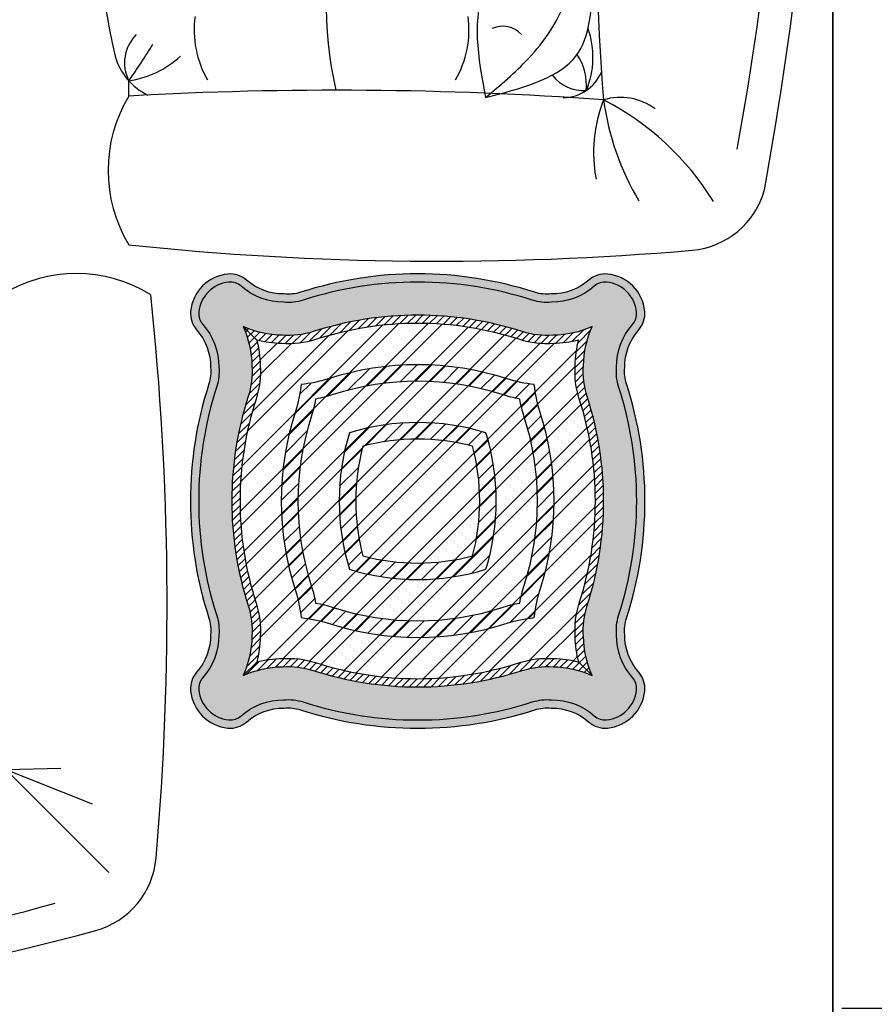
# Model space of a CAD drawing. Units: inches. Extents: x 844 to 2234, y 346 to 1084.
# Tile 67 of 93: x 2014.41 to 2030.9, y 668.63 to 687.63. Entities that reach past the tile are written whole.
import ezdxf

# ---------------------------------------------------------------- set-up
doc = ezdxf.new("R2010")
doc.units = ezdxf.units.IN
doc.header["$MEASUREMENT"] = 0
for name, color, linetype, lineweight in [('A-ANNO-DIMS', 2, 'Continuous', 18), ('A-WALL', 7, 'Continuous', 35), ('furniture', 8, 'Continuous', 18)]:
    doc.layers.add(name, color=color, linetype=linetype, lineweight=lineweight)
for name, color, linetype in [('RA-AP-01$0$FURN', 3, 'Continuous'), ('RA-AP-01$0$steel', 193, 'Continuous'), ('RA-AP-01$0$WOOD', 64, 'Continuous')]:
    doc.layers.add(name, color=color, linetype=linetype)
doc.styles.get("Standard").update_dxf_attribs({"font": 'arial.ttf'})
doc.dimstyles.get("Standard").update_dxf_attribs({"dimtxt": 6, "dimasz": 3, "dimexe": 0.18, "dimexo": 0.0625, "dimgap": 0.09, "dimtad": 0, "dimtih": 1, "dimtoh": 1, "dimdec": 1, "dimzin": 0, "dimdsep": 46, "dimlunit": 3, "dimtxsty": 'Standard', "dimblk": 'ARCHTICK', "dimcen": 0.09, "dimadec": 0, "dimazin": 0, "dimtfac": 1, "dimtdec": 1, "dimtofl": 0, "dimtmove": 0, "dimatfit": 3, "dimfxl": 1, "dimtolj": 1, "dimtzin": 0, "dimarcsym": 0})
pattern_1 = [(45, (0, 1.362436106329781), (-0.0088388347648318, 0.0088388347648318), [])]
pattern_2 = [(45, (0, 1.362436106329781), (-0.0044194173824159, 0.0044194173824159), [])]

# ---------------------------------------------------------------- blocks, each defined once
blk = doc.blocks.new('A$C2FCF5309')
at = {"layer": 'RA-AP-01$0$FURN'}
h = blk.add_hatch(dxfattribs=at)
h.set_pattern_fill('ANSI31', color=256, scale=0.1, style=0)
h.set_pattern_definition(pattern_1)
h.paths.add_polyline_path([(5.038683893313746, -5.169250834004607, -0.1583983521602212), (5.038683893312098, -5.373464580902012, 0.0306258898943267), (5.033304057242972, -5.394827569605182, 0.0306258898948892), (5.01194106853941, -5.40020740567441, -0.1028142994996694), (4.878286182323899, -5.414871334512708), (4.863600873530158, -5.43331743520547, 0.1120482678681049), (5.018059823131753, -5.419248541734471, -0.052642197802937), (5.050972078299936, -5.412495590662115, -0.0526421977994963), (5.057725029371615, -5.379583335496025, 0.1583028414702701), (5.057725029372958, -5.163132079409654, -0.052642197806903), (5.050972078299777, -5.130219824239078, -0.0526421977995126), (5.018059823133679, -5.123466873167369, 0.0215995840215353), (4.988903013548211, -5.115372132362452), (4.975007495303644, -5.132826183367946, -0.0289147572844802), (5.011941068537408, -5.142508009226167, 0.0306258898976746), (5.033304057242868, -5.147887845296027, 0.0306258899022411)])
h.paths.add_polyline_path([(4.975007495303645, -5.132826183367946), (4.988903013548211, -5.115372132362452, 0.1362374241599938), (4.801608567045604, -5.12346687316654, -0.0526421978036853), (4.768696311876971, -5.130219824239102, -0.05264219780204), (4.761943360804856, -5.163132079406747, 0.1583028414743723), (4.761943360806116, -5.379583335498449, -0.0526421977955461), (4.768696311877141, -5.412495590662114, -0.0526421978073986), (4.801608567048022, -5.419248541735437, 0.0454484293938888), (4.863600873530158, -5.43331743520547), (4.878286182323899, -5.414871334512708, -0.0546933379798044), (4.80772732164382, -5.40020740567649, 0.030625889903973), (4.786364332934043, -5.394827569605216, 0.0306258898932853), (4.780984496865101, -5.373464580902791, -0.1583983521638281), (4.780984496864308, -5.169250834000963, 0.03062588989692), (4.786364332933943, -5.147887845296004, 0.0306258898946324), (4.807727321637318, -5.142508009226805, -0.1288932573266927)])
h.paths.add_polyline_path([(4.843422214712861, -5.204945727074827, -0.0783685831716868), (4.924134454130224, -5.196727409635105), (4.939146578618322, -5.177870798323143, 0.1012675676854134), (4.827248748758957, -5.188772261120899, 0.1253648873081696), (4.820394258584192, -5.327034652050361), (4.837127701354095, -5.306015906404253, -0.0981593964869636)], flags=17)
h.paths.add_polyline_path([(4.843422214712824, -5.337769687826355, -0.0311091841722656), (4.837127701354095, -5.306015906404253), (4.820394258584193, -5.32703465205036, 0.0247727657431944), (4.827248748758908, -5.353943153780261, 0.0812754385032542), (4.916962478476905, -5.36629034358622), (4.933684093813825, -5.345286454285511, -0.0876255421014372)], flags=17)
h.paths.add_polyline_path([(4.992419641418037, -5.353943153780226, 0.1506053783834298), (4.992419641417933, -5.188772261120954, 0.0485966419124224), (4.939146578618321, -5.177870798323143), (4.924134454130224, -5.196727409635105, -0.0507799419579301), (4.976246175464031, -5.204945727074882, -0.1296645318906876), (4.97624617546411, -5.337769687826316, -0.0415667119298777), (4.933684093813825, -5.345286454285511), (4.916962478476905, -5.36629034358622, 0.0684915676023693)], flags=17)
h = blk.add_hatch(dxfattribs=at)
h.set_pattern_fill('ANSI31', color=256, scale=0.1, style=0)
h.set_pattern_definition(pattern_1)
h.paths.add_polyline_path([(5.038683893313746, -5.169250834004607, -0.1583983521602212), (5.038683893312098, -5.373464580902012, 0.0306258898943267), (5.033304057242972, -5.394827569605182, 0.0306258898948892), (5.01194106853941, -5.40020740567441, -0.1028142994996694), (4.878286182323899, -5.414871334512708), (4.863600873530158, -5.43331743520547, 0.1120482678681049), (5.018059823131753, -5.419248541734471, -0.052642197802937), (5.050972078299936, -5.412495590662115, -0.0526421977994963), (5.057725029371615, -5.379583335496025, 0.1583028414702701), (5.057725029372958, -5.163132079409654, -0.052642197806903), (5.050972078299777, -5.130219824239078, -0.0526421977995126), (5.018059823133679, -5.123466873167369, 0.0215995840215353), (4.988903013548211, -5.115372132362452), (4.975007495303644, -5.132826183367946, -0.0289147572844802), (5.011941068537408, -5.142508009226167, 0.0306258898976746), (5.033304057242868, -5.147887845296027, 0.0306258899022411)])
h.paths.add_polyline_path([(4.975007495303645, -5.132826183367946), (4.988903013548211, -5.115372132362452, 0.1362374241599938), (4.801608567045604, -5.12346687316654, -0.0526421978036853), (4.768696311876971, -5.130219824239102, -0.05264219780204), (4.761943360804856, -5.163132079406747, 0.1583028414743723), (4.761943360806116, -5.379583335498449, -0.0526421977955461), (4.768696311877141, -5.412495590662114, -0.0526421978073986), (4.801608567048022, -5.419248541735437, 0.0454484293938888), (4.863600873530158, -5.43331743520547), (4.878286182323899, -5.414871334512708, -0.0546933379798044), (4.80772732164382, -5.40020740567649, 0.030625889903973), (4.786364332934043, -5.394827569605216, 0.0306258898932853), (4.780984496865101, -5.373464580902791, -0.1583983521638281), (4.780984496864308, -5.169250834000963, 0.03062588989692), (4.786364332933943, -5.147887845296004, 0.0306258898946324), (4.807727321637318, -5.142508009226805, -0.1288932573266927)])
h.paths.add_polyline_path([(4.843422214712861, -5.204945727074827, -0.0783685831716868), (4.924134454130224, -5.196727409635105), (4.939146578618322, -5.177870798323143, 0.1012675676854134), (4.827248748758957, -5.188772261120899, 0.1253648873081696), (4.820394258584192, -5.327034652050361), (4.837127701354095, -5.306015906404253, -0.0981593964869636)], flags=17)
h.paths.add_polyline_path([(4.843422214712824, -5.337769687826355, -0.0311091841722656), (4.837127701354095, -5.306015906404253), (4.820394258584193, -5.32703465205036, 0.0247727657431944), (4.827248748758908, -5.353943153780261, 0.0812754385032542), (4.916962478476905, -5.36629034358622), (4.933684093813825, -5.345286454285511, -0.0876255421014372)], flags=17)
h.paths.add_polyline_path([(4.992419641418037, -5.353943153780226, 0.1506053783834298), (4.992419641417933, -5.188772261120954, 0.0485966419124224), (4.939146578618321, -5.177870798323143), (4.924134454130224, -5.196727409635105, -0.0507799419579301), (4.976246175464031, -5.204945727074882, -0.1296645318906876), (4.97624617546411, -5.337769687826316, -0.0415667119298777), (4.933684093813825, -5.345286454285511), (4.916962478476905, -5.36629034358622, 0.0684915676023693)], flags=17)
at = {"layer": 'RA-AP-01$0$WOOD'}
h = blk.add_hatch(color=256, dxfattribs=at)
edge = h.paths.add_edge_path()
edge.add_arc((4.683001772622394, -5.026441828662609), 0.0299999999999998, 48.77105092035535, 95.25687599427813)
edge.add_arc((4.684834195088484, -5.046357707450686), 0.0499999999998897, 95.25687599443106, 174.7431240064049)
edge.add_arc((4.664918316300367, -5.044525284985046), 0.0300000000000005, 174.7431240062535, 221.2289490796905)
edge.add_arc((4.591236830209155, -5.109094338216345), 0.0679700159630267, -0.5333070513215148, 41.228949079691915, ccw=False)
edge.add_arc((4.609451302807284, -5.114694777173187), 0.0500000000000008, -17.3556839752095, 5.7020707654044145, ccw=False)
edge.add_arc((5.095208119646659, -5.271357707450659), 0.4603971832811796, 162.0683908477609, 197.9316091523306)
edge.add_arc((4.609451302807533, -5.428020637728902), 0.0500000000000006, -5.702070765320514, 17.355683975293914, ccw=False)
edge.add_arc((4.591236830209412, -5.433621076685779), 0.0679700159630261, -41.228949079600625, 0.5333070514128053, ccw=False)
edge.add_arc((4.664918316300727, -5.498190129916959), 0.0299999999999995, 138.7710509204022, 185.256875994324)
edge.add_arc((4.684834195088642, -5.496357707450695), 0.0499999999997451, 185.2568759946742, 264.74312400432)
edge.add_arc((4.683001772622394, -5.516273586238612), 0.03, 264.743124003969, 311.2289490796446)
edge.add_arc((4.747570825853633, -5.589955072329876), 0.0679700159630271, 89.4666929486321, 131.2289490796457, ccw=False)
edge.add_arc((4.753171264810493, -5.57174059973175), 0.0500000000000015, 72.64431602474701, 95.70207076536133, ccw=False)
edge.add_arc((4.909834195088355, -5.085983782892503), 0.4603971832811774, 252.0683908477147, 287.9316091522845)
edge.add_arc((5.06649712536621, -5.57174059973175), 0.0499999999999999, 84.29792923463953, 107.35568397525361, ccw=False)
edge.add_arc((5.072097564323069, -5.589955072329877), 0.0679700159630274, 48.771050920354185, 90.5333070513679, ccw=False)
edge.add_arc((5.136666617554309, -5.516273586238614), 0.0299999999999997, 228.771050920353, 275.2568759942969)
edge.add_arc((5.134834195088338, -5.496357707450417), 0.0499999999999982, 275.2568759942949, 354.7431240057633)
edge.add_arc((5.154750073876535, -5.498190129916372), 0.0299999999999999, 354.7431240057662, 401.2289490796891)
edge.add_arc((5.228431559967749, -5.433621076685074), 0.0679700159630274, 179.4666929486771, 221.2289490796903, ccw=False)
edge.add_arc((5.210217087369615, -5.428020637728227), 0.0499999999999976, 162.6443160247947, 185.7020707654089, ccw=False)
edge.add_arc((4.724460270530244, -5.271357707450757), 0.4603971832811793, 342.0683908477607, 377.9316091523305)
edge.add_arc((5.210217087369368, -5.114694777172509), 0.0500000000000019, 174.2979292346878, 197.355683975302, ccw=False)
edge.add_arc((5.228431559967489, -5.109094338215639), 0.0679700159630279, 138.7710509203993, 180.5333070514128, ccw=False)
edge.add_arc((5.154750073876174, -5.044525284984457), 0.0300000000000001, 318.771050920401, 365.2568759954636)
edge.add_arc((5.13483419508816, -5.046357707450624), 0.0499999999998349, 5.256875995237118, 84.74312400549572)
edge.add_arc((5.136666617554308, -5.026441828662608), 0.0299999999999994, 84.74312400572185, 131.2289490796446)
edge.add_arc((5.072097564323072, -4.952760342571343), 0.0679700159630261, 269.4666929486298, 311.22894907964354, ccw=False)
edge.add_arc((5.066497125366206, -4.97097481516947), 0.0499999999999992, 252.64431602475162, 275.70207076536565, ccw=False)
edge.add_arc((4.909834195088355, -5.456731632008717), 0.4603971832811764, 72.06839084771546, 107.9316091522853)
edge.add_arc((4.753171264810493, -4.970974815169471), 0.0500000000000016, 264.2979292346387, 287.355683975253, ccw=False)
edge.add_arc((4.747570825853633, -4.952760342571346), 0.0679700159630274, 228.7710509203543, 270.5333070513679, ccw=False)
edge = h.paths.add_edge_path(flags=16)
edge.add_arc((4.683001772622395, -5.026441828662608), 0.019999999999999, 48.7710509203555, 95.2568759942793)
edge.add_arc((4.684834195088469, -5.046357707450671), 0.0399999999998731, 95.2568759944489, 174.7431240064248)
edge.add_arc((4.664918316300404, -5.044525284985035), 0.020000000000036, 174.7431240062186, 221.2289490796461)
edge.add_arc((4.591236830209151, -5.109094338216346), 0.0779700159630296, -0.13764630038667747, 41.228949079689585, ccw=False)
edge.add_arc((4.609451302807307, -5.11469477717304), 0.060000000000024, -17.406127045137907, 5.176192161068002, ccw=False)
edge.add_arc((5.09520811964665, -5.271357707450659), 0.4503971832811708, 162.0623235129628, 197.9376764869162)
edge.add_arc((4.609451302807532, -5.428020637728943), 0.0599999999999982, -5.176192160466428, 17.406127046715312, ccw=False)
edge.add_arc((4.591236830209414, -5.433621076685778), 0.0779700159630257, -41.2289490796029, 0.13764630095249686, ccw=False)
edge.add_arc((4.664918316300731, -5.498190129916961), 0.0200000000000047, 138.7710509204103, 185.2568759943212)
edge.add_arc((4.684834195088606, -5.496357707450731), 0.0399999999997066, 185.2568759947174, 264.7431240043665)
edge.add_arc((4.683001772622369, -5.516273586238541), 0.020000000000069, 264.7431240038842, 311.2289490795622)
edge.add_arc((4.747570825853635, -5.589955072329884), 0.0779700159630344, 89.8623536987642, 131.2289490796432, ccw=False)
edge.add_arc((4.753171264810603, -5.571740599731771), 0.0599999999999895, 72.5938729544394, 95.1761921602253, ccw=False)
edge.add_arc((4.909834195088365, -5.085983782892505), 0.4503971832811724, 252.0623235129989, 287.9376764870498)
edge.add_arc((5.066497125366216, -5.571740599731755), 0.0600000000000047, 84.8238078399923, 107.40612704528041, ccw=False)
edge.add_arc((5.072097564322998, -5.589955072329853), 0.077970015963056, 48.771050920303594, 90.13764630126451, ccw=False)
edge.add_arc((5.136666617554307, -5.516273586238622), 0.0199999999999931, 228.771050920344, 275.2568759943037)
edge.add_arc((5.134834195088338, -5.496357707450416), 0.0400000000000004, 275.2568759942928, 354.7431240057607)
edge.add_arc((5.154750073876533, -5.498190129916375), 0.0200000000000037, 354.7431240057783, 401.2289490796939)
edge.add_arc((5.228431559967745, -5.433621076685076), 0.0779700159630239, 179.8623536995147, 221.2289490796908, ccw=False)
edge.add_arc((5.210217087369586, -5.428020637728345), 0.0600000000000054, 162.5938729554486, 185.1761921609759, ccw=False)
edge.add_arc((4.724460270530243, -5.271357707450766), 0.4503971832811826, 342.0623235128896, 377.937676486982)
edge.add_arc((5.210217087369347, -5.114694777172486), 0.0599999999999777, 174.8238078387611, 197.4061270462219, ccw=False)
edge.add_arc((5.228431559967523, -5.109094338215542), 0.0779700159629885, 138.7710509204687, 180.1376463004423, ccw=False)
edge.add_arc((5.154750073876175, -5.044525284984459), 0.0199999999999989, 318.771050920406, 365.2568759954698)
edge.add_arc((5.134834195088138, -5.046357707450646), 0.0399999999998586, 5.256875995208452, 84.74312400546732)
edge.add_arc((5.136666617554292, -5.02644182866256), 0.0199999999999529, 84.74312400577769, 131.2289490797025)
edge.add_arc((5.072097564323069, -4.952760342571338), 0.077970015963032, 269.86235369901414, 311.2289490796421, ccw=False)
edge.add_arc((5.06649712536618, -4.97097481516946), 0.0600000000000007, 252.5938729548277, 275.17619216047467, ccw=False)
edge.add_arc((4.909834195088353, -5.456731632008716), 0.4503971832811739, 72.06232351293887, 107.9376764867365)
edge.add_arc((4.753171264810429, -4.970974815169467), 0.0599999999999991, 264.82380783985815, 287.40612704769893, ccw=False)
edge.add_arc((4.747570825853681, -4.952760342571361), 0.0779700159630467, 228.7710509203206, 270.13764630113724, ccw=False)
h = blk.add_hatch(color=256, dxfattribs=at)
edge = h.paths.add_edge_path()
edge.add_arc((4.683001772622395, -5.026441828662608), 0.019999999999999, 48.7710509203555, 95.2568759942793)
edge.add_arc((4.684834195088469, -5.046357707450671), 0.0399999999998731, 95.2568759944489, 174.7431240064248)
edge.add_arc((4.664918316300404, -5.044525284985035), 0.020000000000036, 174.7431240062186, 221.2289490796461)
edge.add_arc((4.591236830209151, -5.109094338216346), 0.0779700159630296, -0.13764630038667747, 41.228949079689585, ccw=False)
edge.add_arc((4.609451302807307, -5.11469477717304), 0.060000000000024, -17.406127045137907, 5.176192161068002, ccw=False)
edge.add_arc((5.09520811964665, -5.271357707450659), 0.4503971832811708, 162.0623235129628, 197.9376764869162)
edge.add_arc((4.609451302807532, -5.428020637728943), 0.0599999999999982, -5.176192160466428, 17.406127046715312, ccw=False)
edge.add_arc((4.591236830209414, -5.433621076685778), 0.0779700159630257, -41.2289490796029, 0.13764630095249686, ccw=False)
edge.add_arc((4.664918316300731, -5.498190129916961), 0.0200000000000047, 138.7710509204103, 185.2568759943212)
edge.add_arc((4.684834195088606, -5.496357707450731), 0.0399999999997066, 185.2568759947174, 264.7431240043665)
edge.add_arc((4.683001772622369, -5.516273586238541), 0.020000000000069, 264.7431240038842, 311.2289490795622)
edge.add_arc((4.747570825853635, -5.589955072329884), 0.0779700159630344, 89.8623536987642, 131.2289490796432, ccw=False)
edge.add_arc((4.753171264810603, -5.571740599731771), 0.0599999999999895, 72.5938729544394, 95.1761921602253, ccw=False)
edge.add_arc((4.909834195088365, -5.085983782892505), 0.4503971832811724, 252.0623235129989, 287.9376764870498)
edge.add_arc((5.066497125366216, -5.571740599731755), 0.0600000000000047, 84.8238078399923, 107.40612704528041, ccw=False)
edge.add_arc((5.072097564322998, -5.589955072329853), 0.077970015963056, 48.771050920303594, 90.13764630126451, ccw=False)
edge.add_arc((5.136666617554307, -5.516273586238622), 0.0199999999999931, 228.771050920344, 275.2568759943037)
edge.add_arc((5.134834195088338, -5.496357707450416), 0.0400000000000004, 275.2568759942928, 354.7431240057607)
edge.add_arc((5.154750073876533, -5.498190129916375), 0.0200000000000037, 354.7431240057783, 401.2289490796939)
edge.add_arc((5.228431559967745, -5.433621076685076), 0.0779700159630239, 179.8623536995147, 221.2289490796908, ccw=False)
edge.add_arc((5.210217087369586, -5.428020637728345), 0.0600000000000054, 162.5938729554486, 185.1761921609759, ccw=False)
edge.add_arc((4.724460270530243, -5.271357707450766), 0.4503971832811826, 342.0623235128896, 377.937676486982)
edge.add_arc((5.210217087369347, -5.114694777172486), 0.0599999999999777, 174.8238078387611, 197.4061270462219, ccw=False)
edge.add_arc((5.228431559967523, -5.109094338215542), 0.0779700159629885, 138.7710509204687, 180.1376463004423, ccw=False)
edge.add_arc((5.154750073876175, -5.044525284984459), 0.0199999999999989, 318.771050920406, 365.2568759954698)
edge.add_arc((5.134834195088138, -5.046357707450646), 0.0399999999998586, 5.256875995208452, 84.74312400546732)
edge.add_arc((5.136666617554292, -5.02644182866256), 0.0199999999999529, 84.74312400577769, 131.2289490797025)
edge.add_arc((5.072097564323069, -4.952760342571338), 0.077970015963032, 269.86235369901414, 311.2289490796421, ccw=False)
edge.add_arc((5.06649712536618, -4.97097481516946), 0.0600000000000007, 252.5938729548277, 275.17619216047467, ccw=False)
edge.add_arc((4.909834195088353, -5.456731632008716), 0.4503971832811739, 72.06232351293887, 107.9376764867365)
edge.add_arc((4.753171264810429, -4.970974815169467), 0.0599999999999991, 264.82380783985815, 287.40612704769893, ccw=False)
edge.add_arc((4.747570825853681, -4.952760342571361), 0.0779700159630467, 228.7710509203206, 270.13764630113724, ccw=False)
edge = h.paths.add_edge_path(flags=16)
edge.add_arc((4.591236830209151, -5.109094338216348), 0.1179700159630308, 0.7417751874182841, 24.563326950263672, ccw=False)
edge.add_arc((4.609451302807302, -5.114694777173093), 0.100000000000012, -17.52836504564658, 4.087328884225087, ccw=False)
edge.add_arc((5.095208119646651, -5.271357707450657), 0.4103971832811724, 162.0403002448777, 197.9596997550675)
edge.add_arc((4.60945130280753, -5.428020637728918), 0.1000000000000027, -4.087328883827581, 17.528365046291924, ccw=False)
edge.add_arc((4.591236830209414, -5.433621076685779), 0.1179700159630246, 335.43667305041845, 359.2582248129738, ccw=False)
edge.add_arc((4.747570825853596, -5.589955072329891), 0.117970015963042, 90.7417751868461, 114.5633269496104, ccw=False)
edge.add_arc((4.753171264810559, -5.571740599731767), 0.0999999999999976, 72.47163495370341, 94.0873288836737, ccw=False)
edge.add_arc((4.909834195088367, -5.085983782892503), 0.4103971832811735, 252.0403002449999, 287.9596997551833)
edge.add_arc((5.066497125366205, -5.571740599731755), 0.1000000000000057, 85.91267111645209, 107.5283650455624, ccw=False)
edge.add_arc((5.072097564322985, -5.58995507232986), 0.117970015963046, 65.4366730497672, 89.25822481317113, ccw=False)
edge.add_arc((5.22843155996773, -5.433621076684992), 0.1179700159630096, 180.7417751873964, 204.5633269502712, ccw=False)
edge.add_arc((5.210217087369591, -5.428020637728301), 0.0999999999999969, 162.4716349546276, 184.0873288841682, ccw=False)
edge.add_arc((4.724460270530243, -5.271357707450766), 0.4103971832811825, 342.0403002448147, 377.9596997550345)
edge.add_arc((5.210217087369347, -5.114694777172489), 0.0999999999999796, 175.9126711156995, 197.5283650464392, ccw=False)
edge.add_arc((5.228431559967512, -5.109094338215525), 0.1179700159630019, 155.4366730502992, 179.2582248126247, ccw=False)
edge.add_arc((5.072097564323172, -4.952760342571314), 0.1179700159630537, 270.74177518697286, 294.56332694975765, ccw=False)
edge.add_arc((5.066497125366189, -4.970974815169462), 0.1000000000000017, 252.471634954247, 274.0873288838353, ccw=False)
edge.add_arc((4.909834195088353, -5.456731632008716), 0.4103971832811758, 72.04030024486342, 107.9596997549354)
edge.add_arc((4.75317126481046, -4.970974815169467), 0.1000000000000041, 265.91267111635307, 287.5283650466103, ccw=False)
edge.add_arc((4.747570825853629, -4.952760342571342), 0.1179700159630538, 245.43667304992562, 269.2582248131125, ccw=False)
h = blk.add_hatch(dxfattribs=at)
h.set_pattern_fill('ANSI31', color=256, scale=0.05, style=0)
h.set_pattern_definition(pattern_2)
h.paths.add_polyline_path([(5.105336294329346, -5.394854099602528, 0.0940138826956367), (5.100476366643778, -5.435568764288975, 0.0606271852326483), (5.104678567100611, -5.466202079462671, 0.0606271852344644), (5.074045251925975, -5.46199987900586, 0.0940138827021426), (5.033330587236848, -5.466859806692645, -0.1305325492494615), (4.828072633169377, -5.477944178050054), (4.821119726105699, -5.486677669841435, 0.1336226599878005), (5.036379334063467, -5.476383803188216, -0.0945969211935747), (5.073624810952389, -5.471994942692536, -0.1043170707892296), (5.121137550891356, -5.48266106325342, -0.1043170707868944), (5.110471430330457, -5.435148323315565, -0.0945969211952573), (5.114860290825935, -5.397902846425963, 0.1580239521433527), (5.114860290826324, -5.144812568476775, -0.0945969212010491), (5.110471430330247, -5.10756709158498, -0.1043170707844371), (5.121137550890657, -5.060054351648168, -0.104317070786514), (5.073624810952866, -5.070720472208642, -0.0945969211958523), (5.036379334063063, -5.066331611712874, 0.1580239521426795), (4.783289056114906, -5.066331611712465, -0.0945969211985319), (4.746043579224103, -5.070720472208672, -0.1043170707882665), (4.698530839285552, -5.060054351647925, -0.1043170707867205), (4.709196959846443, -5.10756709158571, -0.094596921196788), (4.704808099350826, -5.144812568475902, 0.1580239521433127), (4.704808099350699, -5.397902846425022, -0.094596921197841), (4.709196959846712, -5.435148323315576, -0.1043170707855109), (4.698530839286393, -5.482661063252921, -0.1043170707864168), (4.746043579224162, -5.471994942692571, -0.0945969211977586), (4.783289056114671, -5.476383803188671, 0.0238966994662183), (4.821119726105699, -5.486677669841435), (4.828072633169378, -5.477944178050054, -0.0269814195959459), (4.786337802940177, -5.466859806692736, 0.0940138827039629), (4.745623138250268, -5.461999879005895, 0.0606271852320776), (4.714989823076826, -5.466202079462476, 0.0606271852304618), (4.719192023533341, -5.435568764289856, 0.0940138826917763), (4.714332095848404, -5.394854099604977, -0.1580706864542086), (4.714332095846561, -5.147861315302034, 0.0940138827032017), (4.719192023533127, -5.107146650612438, 0.0606271852329446), (4.714989823076289, -5.076513335438588, 0.0606271852340035), (4.745623138250698, -5.08071553589536, 0.0940138827025969), (4.786337802940015, -5.075855608208526, -0.1580706864508517), (5.033330587237968, -5.075855608208939, 0.0940138827009578), (5.074045251926627, -5.080715535895319, 0.0606271852322557), (5.104678567100159, -5.076513335438697, 0.0606271852308743), (5.100476366643561, -5.107146650611519, 0.0940138827178109), (5.105336294331983, -5.147861315307182, -0.1580706864490946)])
h = blk.add_hatch(dxfattribs=at)
h.set_pattern_fill('ANSI31', color=256, scale=0.05, style=0)
h.set_pattern_definition(pattern_2)
h.paths.add_polyline_path([(5.105336294329346, -5.394854099602528, 0.0940138826956367), (5.100476366643778, -5.435568764288975, 0.0606271852326483), (5.104678567100611, -5.466202079462671, 0.0606271852344644), (5.074045251925975, -5.46199987900586, 0.0940138827021426), (5.033330587236848, -5.466859806692645, -0.1305325492494615), (4.828072633169377, -5.477944178050054), (4.821119726105699, -5.486677669841435, 0.1336226599878005), (5.036379334063467, -5.476383803188216, -0.0945969211935747), (5.073624810952389, -5.471994942692536, -0.1043170707892296), (5.121137550891356, -5.48266106325342, -0.1043170707868944), (5.110471430330457, -5.435148323315565, -0.0945969211952573), (5.114860290825935, -5.397902846425963, 0.1580239521433527), (5.114860290826324, -5.144812568476775, -0.0945969212010491), (5.110471430330247, -5.10756709158498, -0.1043170707844371), (5.121137550890657, -5.060054351648168, -0.104317070786514), (5.073624810952866, -5.070720472208642, -0.0945969211958523), (5.036379334063063, -5.066331611712874, 0.1580239521426795), (4.783289056114906, -5.066331611712465, -0.0945969211985319), (4.746043579224103, -5.070720472208672, -0.1043170707882665), (4.698530839285552, -5.060054351647925, -0.1043170707867205), (4.709196959846443, -5.10756709158571, -0.094596921196788), (4.704808099350826, -5.144812568475902, 0.1580239521433127), (4.704808099350699, -5.397902846425022, -0.094596921197841), (4.709196959846712, -5.435148323315576, -0.1043170707855109), (4.698530839286393, -5.482661063252921, -0.1043170707864168), (4.746043579224162, -5.471994942692571, -0.0945969211977586), (4.783289056114671, -5.476383803188671, 0.0238966994662183), (4.821119726105699, -5.486677669841435), (4.828072633169378, -5.477944178050054, -0.0269814195959459), (4.786337802940177, -5.466859806692736, 0.0940138827039629), (4.745623138250268, -5.461999879005895, 0.0606271852320776), (4.714989823076826, -5.466202079462476, 0.0606271852304618), (4.719192023533341, -5.435568764289856, 0.0940138826917763), (4.714332095848404, -5.394854099604977, -0.1580706864542086), (4.714332095846561, -5.147861315302034, 0.0940138827032017), (4.719192023533127, -5.107146650612438, 0.0606271852329446), (4.714989823076289, -5.076513335438588, 0.0606271852340035), (4.745623138250698, -5.08071553589536, 0.0940138827025969), (4.786337802940015, -5.075855608208526, -0.1580706864508517), (5.033330587237968, -5.075855608208939, 0.0940138827009578), (5.074045251926627, -5.080715535895319, 0.0606271852322557), (5.104678567100159, -5.076513335438697, 0.0606271852308743), (5.100476366643561, -5.107146650611519, 0.0940138827178109), (5.105336294331983, -5.147861315307182, -0.1580706864490946)])
h = blk.add_hatch(dxfattribs=at)
h.set_pattern_fill('ANSI32,_I', color=256, scale=0.1, style=2)
h.set_pattern_definition([(45, (0, 0), (-0.0265165042944955, 0.0265165042944955), []), (45, (0.0176776695, 0), (-0.0265165042944955, 0.0265165042944955), [])])
h.paths.add_polyline_path([(4.843422214712824, -5.337769687826354, 0.1296645318905289), (4.97624617546411, -5.337769687826316, 0.1296645318906876), (4.976246175464032, -5.204945727074882, 0.129664531890418), (4.843422214712861, -5.204945727074827, 0.129664531890765)], flags=0)
h.paths.add_polyline_path([(5.039131224122924, -5.170637849998464, -0.0326520429852175), (5.033304057242868, -5.147887845296027, -0.0326520429894721), (5.010554052537512, -5.142060678415043, 0.1561383235202698), (4.809114337641437, -5.142060678414318, -0.0326520429925972), (4.786364332933944, -5.147887845296004, -0.0326520429914489), (4.780537166052582, -5.170637850002729, 0.1561383235189577), (4.780537166052134, -5.37207756489719, -0.0326520429934175), (4.786364332934042, -5.394827569605215, -0.0326520429823496), (4.809114337634529, -5.400654736484653, 0.156138323524066), (5.010554052535268, -5.400654736486903, -0.032652042992888), (5.033304057242972, -5.394827569605183, -0.0326520429928733), (5.039131224124712, -5.372077564897496, 0.1561383235226786)], flags=0)
h.paths.add_polyline_path([(4.992419641418037, -5.353943153780226, -0.1506053783832862), (4.827248748758909, -5.353943153780261, -0.1506053783835069), (4.827248748758957, -5.188772261120899, -0.1506053783831346), (4.992419641417933, -5.188772261120954, -0.1506053783834298)], flags=0)
h.paths.add_polyline_path([(4.976246175464111, -5.337769687826316, -0.1296645318905298), (4.843422214712824, -5.337769687826354, -0.129664531890765), (4.843422214712862, -5.204945727074827, -0.1296645318904162), (4.976246175464031, -5.204945727074882, -0.1296645318906876)], flags=0)
h.paths.add_polyline_path([(5.105721254232479, -5.149054940982025, -0.0968902512052664), (5.100476366643561, -5.107146650611519, -0.0606271852308743), (5.104678567100159, -5.076513335438697, -0.0606271852322574), (5.074045251926626, -5.080715535895319, -0.0968902512197216), (5.032136961550132, -5.075470648304253, 0.1564657949319774), (4.787531428625239, -5.075470648304682, -0.0968902512150626), (4.745623138250699, -5.08071553589536, -0.060627185234009), (4.714989823076288, -5.076513335438587, -0.0606271852329501), (4.719192023533127, -5.10714665061244, -0.0968902512185585), (4.713947135942331, -5.149054940988458, 0.1564657949285579), (4.713947135940853, -5.393660473908259, -0.0968902512319826), (4.71919202353334, -5.435568764289873, -0.0606271852304288), (4.714989823076825, -5.466202079462476, -0.0606271852320811), (4.745623138250269, -5.461999879005895, -0.0968902512162649), (4.787531428625332, -5.467244766596559, 0.1564657949327057), (5.032136961551311, -5.46724476659659, -0.0968902512153659), (5.074045251925975, -5.46199987900586, -0.0606271852344627), (5.10467856710061, -5.466202079462671, -0.0606271852326483), (5.100476366643777, -5.435568764288975, -0.0968902512258216), (5.105721254235559, -5.393660473909953, 0.1564657949340142)])
h.paths.add_polyline_path([(5.057725029371625, -5.379583335495999, 0.0526421977995391), (5.050972078299936, -5.412495590662114, 0.0526421978029782), (5.018059823131728, -5.419248541734479, -0.1583028414681072), (4.801608567048168, -5.419248541735485, 0.0526421978076402), (4.76869631187714, -5.412495590662113, 0.0526421977956189), (4.761943360806101, -5.379583335498404, -0.1583028414743129), (4.761943360804846, -5.163132079406778, 0.0526421978020944), (4.768696311876972, -5.130219824239101, 0.0526421978033651), (4.80160856704541, -5.123466873166602, -0.1583028414716875), (5.018059823133628, -5.123466873167353, 0.0526421977995944), (5.050972078299776, -5.130219824239078, 0.0526421978070423), (5.057725029372986, -5.163132079409739, -0.1583028414701848)], flags=16)
h.paths.add_polyline_path([(5.038683893312112, -5.373464580901968, 0.0306258898943915), (5.033304057242972, -5.394827569605182, 0.0306258898948892), (5.01194106853941, -5.40020740567441, -0.1583983521587032), (4.807727321643864, -5.400207405676503, 0.0306258899040366), (4.786364332934043, -5.394827569605215, 0.0306258898931986), (4.780984496865119, -5.37346458090285, -0.1583983521638542), (4.7809844968643, -5.169250834000989, 0.0306258898969596), (4.786364332933945, -5.147887845296004, 0.0306258898946195), (4.807727321637311, -5.142508009226808, -0.1583983521623412), (5.011941068537318, -5.142508009226139, 0.030625889897807), (5.033304057242868, -5.147887845296028, 0.0306258899020632), (5.038683893313706, -5.169250834004486, -0.1583983521602835)], flags=0)
for p, q in [((4.714989823076289, -5.076513335438588), (4.698530839285552, -5.060054351647925)), ((4.714989823076289, -5.076513335438588), (4.698530839285552, -5.060054351647925)), ((5.104678567100159, -5.076513335438697), (5.121137550890656, -5.060054351648169)), ((5.104678567100159, -5.076513335438697), (5.121137550890656, -5.060054351648169)), ((5.10467856710061, -5.466202079462671), (5.121137550891355, -5.482661063253419)), ((5.10467856710061, -5.466202079462671), (5.121137550891355, -5.482661063253419))]:
    blk.add_line(p, q, dxfattribs=at)
for points in [[(4.702773858784635, -5.003879368495489, 0.2056608120285223), (4.680253138923443, -4.996568010480312, 0.3614336704708569), (4.635044498118043, -5.041776651286372, 0.2056608120263112), (4.642355856133262, -5.064297371147306, -0.1842662638101064), (4.65920390179375, -5.10972699154053, -0.1009492694051416), (4.657174869772992, -5.129609908955028, 0.1577727036674954), (4.657174869773219, -5.41310550594699, -0.1009492694051416), (4.659203901794006, -5.432988423361486, -0.1842662638101064), (4.64235585613359, -5.478418043754737, 0.2056608120285221), (4.635044498118431, -5.500938763615934, 0.3614336704593693), (4.680253138922529, -5.546147404420826, 0.2056608120364936), (4.702773858784635, -5.538836046405732, -0.1842662638101064), (4.748203479177874, -5.52198800074528, -0.1009492694051415), (4.768086396592371, -5.524017032766053, 0.1577727036674954), (5.051581993584332, -5.524017032766055, -0.1009492694051416), (5.071464910998829, -5.521988000745282, -0.1842662638101064), (5.116894531392067, -5.538836046405734, 0.2056608120286145), (5.13941525125327, -5.546147404420911, 0.3614336704683636), (5.184623892058835, -5.500938763615299, 0.2056608120285223), (5.177312534043641, -5.478418043754112, -0.1842662638101063), (5.160464488383153, -5.432988423360887, -0.1009492694051416), (5.162493520403909, -5.41310550594639, 0.1577727036674954), (5.162493520403684, -5.129609908954428, -0.1009492694051416), (5.160464488382894, -5.109726991539933, -0.1842662638101064), (5.17731253404331, -5.064297371146681, 0.2056608120337072), (5.184623892058415, -5.041776651284888, 0.3614336704623863), (5.139415251253259, -4.99656801048031, 0.2056608120285223), (5.116894531392067, -5.003879368495487, -0.1842662638101064), (5.071464910998829, -5.020727414155937, -0.1009492694051416), (5.051581993584332, -5.018698382135166, 0.1577727036674956), (4.768086396592371, -5.018698382135168, -0.1009492694051416), (4.748203479177874, -5.020727414155941, -0.1842662638101064)], [(4.702773858784635, -5.003879368495489, 0.2056608120285223), (4.680253138923443, -4.996568010480312, 0.3614336704708569), (4.635044498118043, -5.041776651286372, 0.2056608120263112), (4.642355856133262, -5.064297371147306, -0.1842662638101064), (4.65920390179375, -5.10972699154053, -0.1009492694051416), (4.657174869772992, -5.129609908955028, 0.1577727036674954), (4.657174869773219, -5.41310550594699, -0.1009492694051416), (4.659203901794006, -5.432988423361486, -0.1842662638101064), (4.64235585613359, -5.478418043754737, 0.2056608120285221), (4.635044498118431, -5.500938763615934, 0.3614336704593693), (4.680253138922529, -5.546147404420826, 0.2056608120364936), (4.702773858784635, -5.538836046405732, -0.1842662638101064), (4.748203479177874, -5.52198800074528, -0.1009492694051415), (4.768086396592371, -5.524017032766053, 0.1577727036674954), (5.051581993584332, -5.524017032766055, -0.1009492694051416), (5.071464910998829, -5.521988000745282, -0.1842662638101064), (5.116894531392067, -5.538836046405734, 0.2056608120286145), (5.13941525125327, -5.546147404420911, 0.3614336704683636), (5.184623892058835, -5.500938763615299, 0.2056608120285223), (5.177312534043641, -5.478418043754112, -0.1842662638101063), (5.160464488383153, -5.432988423360887, -0.1009492694051416), (5.162493520403909, -5.41310550594639, 0.1577727036674954), (5.162493520403684, -5.129609908954428, -0.1009492694051416), (5.160464488382894, -5.109726991539933, -0.1842662638101064), (5.17731253404331, -5.064297371146681, 0.2056608120337072), (5.184623892058415, -5.041776651284888, 0.3614336704623863), (5.139415251253259, -4.99656801048031, 0.2056608120285223), (5.116894531392067, -5.003879368495487, -0.1842662638101064), (5.071464910998829, -5.020727414155937, -0.1009492694051416), (5.051581993584332, -5.018698382135166, 0.1577727036674956), (4.768086396592371, -5.018698382135168, -0.1009492694051416), (4.748203479177874, -5.020727414155941, -0.1842662638101064)], [(4.696183163397222, -5.011400188551196, 0.2056608120285295), (4.681169350156427, -5.006525949874411, 0.3614336704708588), (4.645002437512154, -5.042692862519237, 0.2056608120262659), (4.649876676188964, -5.057706675759887, -0.182481815856965), (4.669206621172843, -5.109281651732388, -0.0988540857970112), (4.666703803477437, -5.13264334722805, 0.1578269695851905), (4.666703803477144, -5.410072067672365, -0.0988540858013112), (4.6692066211731, -5.433433763168966, -0.1824818158591246), (4.649876676189301, -5.485008739142145, 0.2056608120284717), (4.64500243751253, -5.500022552382944, 0.3614336704593821), (4.681169350155757, -5.536189465026749, 0.2056608120365057), (4.696183163397221, -5.531315226350026, -0.1824818158605826), (4.747758139370833, -5.51198528136619, -0.0988540857951607), (4.771119834866025, -5.514488099061806, 0.1578269695856264), (5.04854855531107, -5.514488099061688, -0.0988540857929677), (5.071910250805761, -5.511985281366138, -0.1824818158609529), (5.123485226779481, -5.531315226350027, 0.2056608120286893), (5.138499040020282, -5.536189465026812, 0.3614336704683556), (5.174665952664737, -5.500022552382323, 0.2056608120284882), (5.169791713987938, -5.485008739141532, -0.1824818158574124), (5.150461769004059, -5.4334337631689, -0.0988540857940221), (5.152964586699289, -5.410072067673927, 0.1578269695858123), (5.1529645866996, -5.132643347228565, -0.0988540858025403), (5.150461769003872, -5.109281651731659, -0.1824818158565006), (5.169791713987599, -5.057706675759273, 0.2056608120337192), (5.174665952664335, -5.042692862518078, 0.3614336704623903), (5.138499040020236, -5.006525949874406, 0.2056608120285323), (5.123485226779481, -5.011400188551195, -0.1824818158594503), (5.071910250806212, -5.03073013353503, -0.09885408579455), (5.048548555311143, -5.028227315839558, 0.1578269695844942), (4.771119834867991, -5.028227315838772, -0.0988540858042156), (4.747758139370745, -5.030730133535067, -0.1824818158603032)], [(4.696183163397222, -5.011400188551196, 0.2056608120285295), (4.681169350156427, -5.006525949874411, 0.3614336704708588), (4.645002437512154, -5.042692862519237, 0.2056608120262659), (4.649876676188964, -5.057706675759887, -0.182481815856965), (4.669206621172843, -5.109281651732388, -0.0988540857970112), (4.666703803477437, -5.13264334722805, 0.1578269695851905), (4.666703803477144, -5.410072067672365, -0.0988540858013112), (4.6692066211731, -5.433433763168966, -0.1824818158591246), (4.649876676189301, -5.485008739142145, 0.2056608120284717), (4.64500243751253, -5.500022552382944, 0.3614336704593821), (4.681169350155757, -5.536189465026749, 0.2056608120365057), (4.696183163397221, -5.531315226350026, -0.1824818158605826), (4.747758139370833, -5.51198528136619, -0.0988540857951607), (4.771119834866025, -5.514488099061806, 0.1578269695856264), (5.04854855531107, -5.514488099061688, -0.0988540857929677), (5.071910250805761, -5.511985281366138, -0.1824818158609529), (5.123485226779481, -5.531315226350027, 0.2056608120286893), (5.138499040020282, -5.536189465026812, 0.3614336704683556), (5.174665952664737, -5.500022552382323, 0.2056608120284882), (5.169791713987938, -5.485008739141532, -0.1824818158574124), (5.150461769004059, -5.4334337631689, -0.0988540857940221), (5.152964586699289, -5.410072067673927, 0.1578269695858123), (5.1529645866996, -5.132643347228565, -0.0988540858025403), (5.150461769003872, -5.109281651731659, -0.1824818158565006), (5.169791713987599, -5.057706675759273, 0.2056608120337192), (5.174665952664335, -5.042692862518078, 0.3614336704623903), (5.138499040020236, -5.006525949874406, 0.2056608120285323), (5.123485226779481, -5.011400188551195, -0.1824818158594503), (5.071910250806212, -5.03073013353503, -0.09885408579455), (5.048548555311143, -5.028227315839558, 0.1578269695844942), (4.771119834867991, -5.028227315838772, -0.0988540858042156), (4.747758139370745, -5.030730133535067, -0.1824818158603032)], [(4.698530839285552, -5.060054351647925, -0.1043170707867612), (4.709196959846444, -5.107567091585729, -0.0945969211969405), (4.704808099350802, -5.144812568475978, 0.1580239521432241), (4.704808099350681, -5.397902846424963, -0.0945969211980322), (4.709196959846711, -5.43514832331559, -0.104317070785482), (4.698530839286393, -5.482661063252921, -0.1043170707864036), (4.746043579224155, -5.471994942692571, -0.094596921197375), (4.78328905611452, -5.476383803188623, 0.1580239521431959), (5.036379334063463, -5.476383803188218, -0.0945969211935888), (5.07362481095239, -5.471994942692536, -0.1043170707892253), (5.121137550891355, -5.482661063253419, -0.1043170707868921), (5.110471430330457, -5.435148323315565, -0.0945969211954828), (5.114860290825962, -5.397902846425878, 0.158023952143358), (5.114860290826295, -5.144812568476682, -0.0945969212007617), (5.110471430330247, -5.107567091584995, -0.1043170707844689), (5.121137550890656, -5.060054351648169, -0.1043170707864946), (5.073624810952874, -5.070720472208642, -0.0945969211956941), (5.036379334063131, -5.066331611712896, 0.1580239521426976), (4.783289056114946, -5.066331611712452, -0.0945969211986379), (4.746043579224103, -5.070720472208672, -0.1043170707882684)], [(4.698530839285552, -5.060054351647925, -0.1043170707867612), (4.709196959846444, -5.107567091585729, -0.0945969211969405), (4.704808099350802, -5.144812568475978, 0.1580239521432241), (4.704808099350681, -5.397902846424963, -0.0945969211980322), (4.709196959846711, -5.43514832331559, -0.104317070785482), (4.698530839286393, -5.482661063252921, -0.1043170707864036), (4.746043579224155, -5.471994942692571, -0.094596921197375), (4.78328905611452, -5.476383803188623, 0.1580239521431959), (5.036379334063463, -5.476383803188218, -0.0945969211935888), (5.07362481095239, -5.471994942692536, -0.1043170707892253), (5.121137550891355, -5.482661063253419, -0.1043170707868921), (5.110471430330457, -5.435148323315565, -0.0945969211954828), (5.114860290825962, -5.397902846425878, 0.158023952143358), (5.114860290826295, -5.144812568476682, -0.0945969212007617), (5.110471430330247, -5.107567091584995, -0.1043170707844689), (5.121137550890656, -5.060054351648169, -0.1043170707864946), (5.073624810952874, -5.070720472208642, -0.0945969211956941), (5.036379334063131, -5.066331611712896, 0.1580239521426976), (4.783289056114946, -5.066331611712452, -0.0945969211986379), (4.746043579224103, -5.070720472208672, -0.1043170707882684)], [(4.714989823076289, -5.076513335438588, -0.0606271852329464), (4.719192023533127, -5.107146650612439, -0.0940138827030756), (4.714332095846578, -5.147861315301983, 0.1580706864542707), (4.714332095848417, -5.394854099605018, -0.0940138826916965), (4.719192023533341, -5.435568764289864, -0.0606271852304462), (4.714989823076826, -5.466202079462476, -0.0606271852320585), (4.745623138250258, -5.461999879005895, -0.0940138827037036), (4.786337802940059, -5.466859806692699, 0.1580706864500221), (5.033330587236783, -5.466859806692666, -0.0940138827023111), (5.074045251925979, -5.46199987900586, -0.060627185234454), (5.10467856710061, -5.466202079462671, -0.0606271852326709), (5.100476366643777, -5.435568764288963, -0.0940138826958686), (5.105336294329379, -5.394854099602421, 0.1580706864489859), (5.105336294331999, -5.147861315307237, -0.0940138827179432), (5.100476366643561, -5.107146650611518, -0.0606271852308726), (5.104678567100159, -5.076513335438697, -0.0606271852322592), (5.074045251926625, -5.080715535895319, -0.094013882701022), (5.03333058723794, -5.075855608208931, 0.1580706864508015), (4.786337802940061, -5.075855608208511, -0.0940138827027143), (4.745623138250695, -5.08071553589536, -0.0606271852339983)], [(4.714989823076289, -5.076513335438588, -0.0606271852329464), (4.719192023533127, -5.107146650612439, -0.0940138827030756), (4.714332095846578, -5.147861315301983, 0.1580706864542707), (4.714332095848417, -5.394854099605018, -0.0940138826916965), (4.719192023533341, -5.435568764289864, -0.0606271852304462), (4.714989823076826, -5.466202079462476, -0.0606271852320585), (4.745623138250258, -5.461999879005895, -0.0940138827037036), (4.786337802940059, -5.466859806692699, 0.1580706864500221), (5.033330587236783, -5.466859806692666, -0.0940138827023111), (5.074045251925979, -5.46199987900586, -0.060627185234454), (5.10467856710061, -5.466202079462671, -0.0606271852326709), (5.100476366643777, -5.435568764288963, -0.0940138826958686), (5.105336294329379, -5.394854099602421, 0.1580706864489859), (5.105336294331999, -5.147861315307237, -0.0940138827179432), (5.100476366643561, -5.107146650611518, -0.0606271852308726), (5.104678567100159, -5.076513335438697, -0.0606271852322592), (5.074045251926625, -5.080715535895319, -0.094013882701022), (5.03333058723794, -5.075855608208931, 0.1580706864508015), (4.786337802940061, -5.075855608208511, -0.0940138827027143), (4.745623138250695, -5.08071553589536, -0.0606271852339983)], [(4.768696311876972, -5.130219824239102, -0.0526421978019087), (4.761943360804882, -5.163132079406667, 0.1583028414744761), (4.761943360806133, -5.379583335498504, -0.0526421977954539), (4.76869631187714, -5.412495590662113, -0.0526421978076619), (4.801608567048181, -5.419248541735488, 0.1583028414681522), (5.0180598231318, -5.419248541734456, -0.0526421978028585), (5.050972078299936, -5.412495590662114, -0.0526421977992923), (5.057725029371576, -5.379583335496149, 0.1583028414703719), (5.057725029372956, -5.163132079409646, -0.0526421978068888), (5.050972078299776, -5.130219824239078, -0.052642197799403), (5.018059823133745, -5.12346687316739, 0.1583028414717216), (4.801608567045482, -5.123466873166579, -0.0526421978034837)], [(4.768696311876972, -5.130219824239102, -0.0526421978019087), (4.761943360804882, -5.163132079406667, 0.1583028414744761), (4.761943360806133, -5.379583335498504, -0.0526421977954539), (4.76869631187714, -5.412495590662113, -0.0526421978076619), (4.801608567048181, -5.419248541735488, 0.1583028414681522), (5.0180598231318, -5.419248541734456, -0.0526421978028585), (5.050972078299936, -5.412495590662114, -0.0526421977992923), (5.057725029371576, -5.379583335496149, 0.1583028414703719), (5.057725029372956, -5.163132079409646, -0.0526421978068888), (5.050972078299776, -5.130219824239078, -0.052642197799403), (5.018059823133745, -5.12346687316739, 0.1583028414717216), (4.801608567045482, -5.123466873166579, -0.0526421978034837)], [(4.786364332933944, -5.147887845296004, -0.0306258898969254), (4.780984496864308, -5.169250834000966, 0.1583983521638412), (4.780984496865107, -5.373464580902811, -0.0306258898932568), (4.786364332934043, -5.394827569605216, -0.0306258899041339), (4.80772732164393, -5.400207405676526, 0.1583983521586416), (5.011941068539401, -5.400207405674413, -0.0306258898949021), (5.033304057242972, -5.394827569605182, -0.0306258898943513), (5.038683893312104, -5.373464580901996, 0.1583983521602784), (5.038683893313717, -5.16925083400452, -0.0306258899021139), (5.033304057242868, -5.147887845296027, -0.030625889897777), (5.011941068537338, -5.142508009226145, 0.1583983521624288), (4.807727321637224, -5.142508009226835, -0.0306258898944937)], [(4.786364332933944, -5.147887845296004, -0.0306258898969254), (4.780984496864308, -5.169250834000966, 0.1583983521638412), (4.780984496865107, -5.373464580902811, -0.0306258898932568), (4.786364332934043, -5.394827569605216, -0.0306258899041339), (4.80772732164393, -5.400207405676526, 0.1583983521586416), (5.011941068539401, -5.400207405674413, -0.0306258898949021), (5.033304057242972, -5.394827569605182, -0.0306258898943513), (5.038683893312104, -5.373464580901996, 0.1583983521602784), (5.038683893313717, -5.16925083400452, -0.0306258899021139), (5.033304057242868, -5.147887845296027, -0.030625889897777), (5.011941068537338, -5.142508009226145, 0.1583983521624288), (4.807727321637224, -5.142508009226835, -0.0306258898944937)], [(4.827248748758957, -5.1887722611209, 0.1506053783835061), (4.827248748758908, -5.353943153780261, 0.150605378383287), (4.992419641418037, -5.353943153780226, 0.1506053783834298), (4.992419641417933, -5.188772261120954, 0.1506053783831346)], [(4.827248748758957, -5.1887722611209, 0.1506053783835061), (4.827248748758908, -5.353943153780261, 0.150605378383287), (4.992419641418037, -5.353943153780226, 0.1506053783834298), (4.992419641417933, -5.188772261120954, 0.1506053783831346)], [(4.843422214712861, -5.204945727074827, 0.1296645318907659), (4.843422214712824, -5.337769687826355, 0.1296645318905299), (4.976246175464111, -5.337769687826316, 0.1296645318906876), (4.976246175464032, -5.204945727074882, 0.129664531890418)], [(4.843422214712861, -5.204945727074827, 0.1296645318907659), (4.843422214712824, -5.337769687826355, 0.1296645318905299), (4.976246175464111, -5.337769687826316, 0.1296645318906876), (4.976246175464032, -5.204945727074882, 0.129664531890418)]]:
    blk.add_lwpolyline(points, format="xyb", close=True, dxfattribs=at)
blk = doc.blocks.new('A$C7EE91E48')
at = {"layer": 'RA-AP-01$0$FURN'}
blk.add_line((7.876483058149153, -8.916612252413607), (7.894824413563697, -8.91661225241228), dxfattribs=at)
for centre, radius, start, end in [((8.2640574776289, -10.44238280163197), 1.579145581857318, 83.41160874364557, 102.4080053169127), ((7.786483058149641, -9.0661122524033), 0.1744999999876311, 58.95177800404691, 121.0482219959532), ((7.945541828320179, -8.972574909806593), 0.0753785023123622, 106.0166452769965, 154.1254380939441), ((7.916754957218176, -8.959417410432842), 0.0479292786975047, 44.59745392834464, 117.1929131456445), ((11.22944555801345, -9.291612252417751), 3.552808610866049, 173.9411276243419, 184.9526687683587), ((3.409601832891398, -9.167687782925107), 4.473931917517753, 355.8522766368882, 3.217109747617342), ((8.01520457216173, -8.897645467382876), 0.1218651776285568, 188.9537679045875, 221.9624470435566), ((8.526336470461455, -8.003664990327692), 1.11020813118073, 235.3335226812019, 238.0671391402286), ((7.956650865392597, -9.11718462924615), 0.1214118203512435, 82.30833671084402, 119.8580925514403), ((7.99288216485019, -9.665283690153952), 0.5100538472773755, 76.6877768646062, 102.3817510640692), ((7.956650865392721, -9.206930729144496), 0.1214118203512435, 240.1419074487191, 277.6916632893155), ((7.929974688293188, -9.369186052387374), 0.0310151388417235, 312.6210548449607, 24.22396814861084), ((7.930919758739578, -9.467332461384675), 0.0478550828899777, 127.3166170761785, 183.424704368466), ((7.924743647870982, -9.442442658911482), 0.05, 180.0000000009465, 247.4173275753961), ((7.889364060496281, -9.40215366480788), 0.0683206773889159, 264.7816049573631, 303.3270138506551), ((7.923648679852059, -9.374174170762846), 0.1042084262671507, 247.1307060672184, 289.5171681282844), ((7.808581237601552, -9.648968385188004), 0.1698955038956699, 68.14876161988033, 101.1221568640549), ((8.0771718498821, -11.93482586084473), 2.452160434589619, 80.15422882944125, 94.80385356032536), ((7.571084966418371, -9.33652322886128), 0.3382138395168437, 301.7436291657352, 332.7696672905972), ((7.915233840274116, -9.812515797398348), 0.3241573581843151, 97.6973649013944, 120.7014325157311), ((7.804376295282986, -9.511725524783945), 0.0704710051510922, 323.5873503842904, 16.86613657946742), ((7.789528504274103, -9.589702786759155), 0.1, 184.9526687683584, 254.500505399143), ((8.57237136322441, -5.436149540861864), 4.284827979137255, 259.7800742526421, 267.8083646714428), ((8.715914569106038, -4.284064429245874), 5.485438776325237, 259.9939267779087, 271.1495965306511)]:
    blk.add_arc(centre, radius, start, end, dxfattribs=at)
for points, knots in [([(7.874668826265334, -9.348473919394923), (7.923124466881221, -9.339303204541801), (7.993324954872194, -9.326017059735285), (8.06376157752081, -9.390102169424527), (8.103134132965852, -9.431527358661508), (8.221004028216989, -9.481194893850247), (8.019427121121076, -9.481144249541355), (7.906405414031112, -9.47017772507408), (7.885651849246296, -9.390591733209991), (7.874668826265335, -9.348473919394923)], [0, 0, 0, 0, 0.1367586589314802, 0.1981301758052378, 0.2677729570689291, 0.3281194902553331, 0.4737578340741574, 0.5765194025309534, 0.692033228742227, 0.692033228742227, 0.692033228742227, 0.692033228742227]), ([(7.874668826265335, -9.348473919394923), (7.889628068095545, -9.36625745808265), (7.922760005094681, -9.405644687068653), (7.98990869426565, -9.453232095877508), (8.07489312913563, -9.45187167035591), (8.127460764320832, -9.46528408601241), (8.154388166447475, -9.472154501784399)], [0, 0, 0, 0, 0.0700185406710163, 0.1550780383534512, 0.2344491945777064, 0.317804873756831, 0.317804873756831, 0.317804873756831, 0.317804873756831])]:
    blk.add_open_spline(points, degree=3, knots=knots, dxfattribs=at)
blk = doc.blocks.new('A$C6E322C05')
at = {"layer": 'RA-AP-01$0$FURN'}
for p, q in [((6.391873508750865, -6.482044957760267), (6.516651486950081, -6.357266979564481)), ((6.391873508750865, -6.482044957760271), (6.43343929223883, -6.37746472106399)), ((6.391873508750866, -6.48204495776027), (6.390422568951521, -6.415535276369585))]:
    blk.add_line(p, q, dxfattribs=at)
for centre, radius, start, end in [((6.192206456970573, -9.839674509409203), 3.552808610866049, 85.0473312316412, 96.0588723756579), ((6.490296991311982, -6.399757455669855), 0.1, 15.49949460085664, 85.04733123164101), ((5.962206456956505, -6.396712009545393), 0.1706604816468166, 148.1725534208377, 211.8274465791593), ((4.33669785707999, -6.99698289606033), 2.33487526667919, 357.3063521928599, 15.49949460085664), ((4.846593614069285, -6.909687157115225), 1.775196618325768, 356.4780136403396, 15.93354743557553)]:
    blk.add_arc(centre, radius, start, end, dxfattribs=at)
blk = doc.blocks.new('A$C5D2F253E')
at = {"layer": 'RA-AP-01$0$FURN', "xscale": -1}
blk.add_blockref('A$C6E322C05', (4.620200485489021, 7.961130550668883), dxfattribs=at)
at = {"layer": 'RA-AP-01$0$steel', "xscale": -1, "rotation": 90}
blk.add_blockref('A$C2FCF5309', (-6.718089885104291, 6.887361125335871), dxfattribs=at)
at = {"layer": 'RA-AP-01$0$WOOD', "xscale": -1, "rotation": 180}
blk.add_blockref('A$C7EE91E48', (-8.833013809079146, -7.288751725733902), dxfattribs=at)
blk = doc.blocks.new('_ArchTick')
at = {"color": 0, "linetype": 'ByBlock', "const_width": 0.15}
blk.add_lwpolyline([(-0.5, -0.5), (0.5, 0.5)], dxfattribs=at)
blk = doc.blocks.new('*D121')
at = {"layer": 'A-ANNO-DIMS', "color": 0, "lineweight": -2, "transparency": 16777216}
for p, q in [((2030.271987351997, 734.262611118704), (2040.245275089302, 734.262611118704)), ((2040.065275089302, 734.262611118704), (2040.065275089302, 704.6043509484256)), ((2040.065275089302, 668.557359536674), (2040.065275089302, 698.2156197069523)), ((2030.271987351997, 668.557359536674), (2040.245275089302, 668.557359536674))]:
    blk.add_line(p, q, dxfattribs=at)
at = {"layer": 'Defpoints', "color": 0, "transparency": 16777216}
for p in [(2030.209487351997, 734.262611118704), (2040.065275089302, 734.262611118704), (2030.209487351997, 668.557359536674)]:
    blk.add_point(p, dxfattribs=at)
at = {"layer": 'A-ANNO-DIMS', "color": 0, "lineweight": -2, "transparency": 16777216, "xscale": 3, "yscale": 3, "zscale": 3}
for p, rotation in [((2040.065275089302, 734.262611118704), 90), ((2040.065275089302, 668.557359536674), 270)]:
    blk.add_blockref('_ArchTick', p, dxfattribs=dict(at, rotation=rotation))
at = {"layer": 'A-ANNO-DIMS', "color": 0, "transparency": 16777216, "insert": (2040.065275089302, 701.4099853276883), "char_height": 6, "attachment_point": 5}
blk.add_mtext('\\A1;LOUNGE SET 5\'-5 1/2" TYP.', dxfattribs=at)

msp = doc.modelspace()

# ---------------------------------------------------------------- linework, layer by layer
at = {"layer": 'A-WALL'}
msp.add_line((2030.099168352677, 766.4551697629895), (2030.099168352677, 629.4551697629895), dxfattribs=at)

# ---------------------------------------------------------------- block references
at = {"layer": 'furniture', "xscale": -15.94108302203742, "yscale": 15.94108302203742, "zscale": 15.94108302203742, "rotation": 270}
msp.add_blockref('A$C5D2F253E', (1990.567271852805, 701.4028671565849), dxfattribs=at)

# ---------------------------------------------------------------- dimensions: what is measured, and where the dimension line sits
at = {"layer": 'A-ANNO-DIMS'}
dim = msp.add_linear_dim(base=(2040.065275089302, 734.262611118704), p1=(2030.209487351996, 668.5573595366737), p2=(2030.209487351996, 734.2626111187037), angle=90, text='LOUNGE SET <> TYP.', dimstyle='Standard', override={"dimdec": 1, "dimlfac": 1, "dimrnd": 0, "dimzin": 1, "dimdsep": 46, "dimlunit": 4, "dimfrac": 2}, dxfattribs=at)
dim.commit()
dim.dimension.update_dxf_attribs({"geometry": '*D121', "text_midpoint": (2040.065275089302, 701.4099853276883)})

doc.saveas('drawing.dxf')
